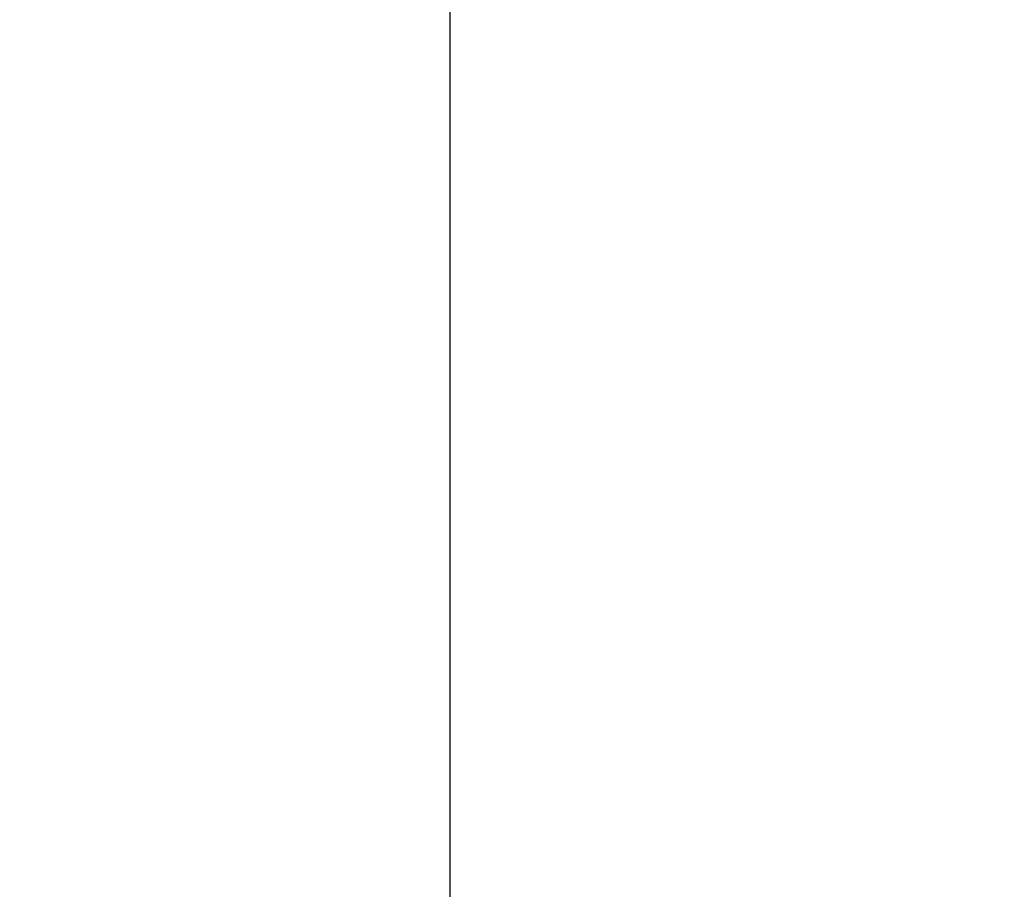
# Model space of a CAD drawing. Units: inches. Extents: x -48 to 50072, y 0 to 21068.
# Tile 21 of 75: x 263 to 341, y 347 to 417. Entities that reach past the tile are written whole.
import ezdxf

# ---------------------------------------------------------------- set-up
doc = ezdxf.new("R2010")
doc.units = ezdxf.units.IN
doc.header["$MEASUREMENT"] = 0
doc.layers.add('A-ANNO-DIMS', color=2, linetype='Continuous', lineweight=18)
doc.styles.get("Standard").update_dxf_attribs({"font": 'arial.ttf'})
doc.dimstyles.get("Standard").update_dxf_attribs({"dimtxt": 8, "dimasz": 0.18, "dimexe": 0.18, "dimexo": 0.0625, "dimgap": 0.09, "dimtad": 0, "dimtih": 1, "dimtoh": 1, "dimdec": 1, "dimzin": 0, "dimdsep": 46, "dimlunit": 4, "dimtxsty": 'Standard', "dimblk": 'ARCHTICK', "dimcen": 0.09, "dimadec": 0, "dimazin": 0, "dimtfac": 1, "dimtdec": 1, "dimtofl": 0, "dimtmove": 0, "dimatfit": 3, "dimldrblk": 'ARCHTICK', "dimfxl": 1, "dimtolj": 1, "dimtzin": 0, "dimarcsym": 0})

# ---------------------------------------------------------------- blocks, each defined once
blk = doc.blocks.new('_ArchTick')
at = {"color": 0, "linetype": 'ByBlock', "const_width": 0.15}
blk.add_lwpolyline([(-0.5, -0.5), (0.5, 0.5)], dxfattribs=at)
blk = doc.blocks.new('*D117')
at = {"layer": 'A-ANNO-DIMS', "color": 0, "lineweight": -2, "transparency": 16777216}
for p, q in [((216.017, 488.712), (216.017, 165.945)), ((297.017, 488.712), (297.017, 165.945)), ((216.017, 166.125), (251.464, 166.125)), ((297.017, 166.125), (261.57, 166.125))]:
    blk.add_line(p, q, dxfattribs=at)
at = {"layer": 'Defpoints', "color": 0, "transparency": 16777216}
for p in [(216.017, 488.775), (297.017, 488.775), (297.017, 166.125)]:
    blk.add_point(p, dxfattribs=at)
at = {"layer": 'A-ANNO-DIMS', "color": 0, "lineweight": -2, "transparency": 16777216, "xscale": 0.18, "yscale": 0.18, "zscale": 0.18, "rotation": 180}
blk.add_blockref('_ArchTick', (216.017, 166.125), dxfattribs=at)
at = {"layer": 'A-ANNO-DIMS', "color": 0, "lineweight": -2, "transparency": 16777216, "xscale": 0.18, "yscale": 0.18, "zscale": 0.18}
blk.add_blockref('_ArchTick', (297.017, 166.125), dxfattribs=at)
at = {"layer": 'A-ANNO-DIMS', "color": 0, "transparency": 16777216, "insert": (256.517, 166.125), "char_height": 8, "attachment_point": 5}
blk.add_mtext('\\A1;81', dxfattribs=at)
blk = doc.blocks.new('*D118')
at = {"layer": 'A-ANNO-DIMS', "color": 0, "lineweight": -2, "transparency": 16777216}
for p, q in [((297.017, 488.712), (297.017, 165.945)), ((463.517, 488.712), (463.517, 165.945)), ((297.017, 166.125), (367.026, 166.125)), ((463.517, 166.125), (393.509, 166.125))]:
    blk.add_line(p, q, dxfattribs=at)
at = {"layer": 'Defpoints', "color": 0, "transparency": 16777216}
for p in [(297.017, 488.775), (463.517, 488.775), (463.517, 166.125)]:
    blk.add_point(p, dxfattribs=at)
at = {"layer": 'A-ANNO-DIMS', "color": 0, "lineweight": -2, "transparency": 16777216, "xscale": 0.18, "yscale": 0.18, "zscale": 0.18, "rotation": 180}
blk.add_blockref('_ArchTick', (297.017, 166.125), dxfattribs=at)
at = {"layer": 'A-ANNO-DIMS', "color": 0, "lineweight": -2, "transparency": 16777216, "xscale": 0.18, "yscale": 0.18, "zscale": 0.18}
blk.add_blockref('_ArchTick', (463.517, 166.125), dxfattribs=at)
at = {"layer": 'A-ANNO-DIMS', "color": 0, "transparency": 16777216, "insert": (380.267, 166.125), "char_height": 8, "attachment_point": 5}
blk.add_mtext('\\A1;166.5', dxfattribs=at)

msp = doc.modelspace()

# ---------------------------------------------------------------- dimensions: what is measured, and where the dimension line sits
at = {"layer": 'A-ANNO-DIMS'}
for base, p1, p2, override, picture, middle in [((297.017, 166.125), (216.017, 488.775), (297.017, 488.775), {"dimdec": 0, "dimlfac": 1, "dimrnd": 0, "dimzin": 0, "dimdsep": 46, "dimlunit": 2}, '*D117', (256.517, 166.125)), ((463.517, 166.125), (297.017, 488.775), (463.517, 488.775), {"dimdec": 1, "dimlfac": 1, "dimrnd": 0, "dimzin": 0, "dimdsep": 46, "dimlunit": 2}, '*D118', (380.267, 166.125))]:
    dim = msp.add_linear_dim(base=base, p1=p1, p2=p2, dimstyle='Standard', override=override, dxfattribs=at)
    dim.commit()
    dim.dimension.update_dxf_attribs({"geometry": picture, "text_midpoint": middle})

doc.saveas('drawing.dxf')
